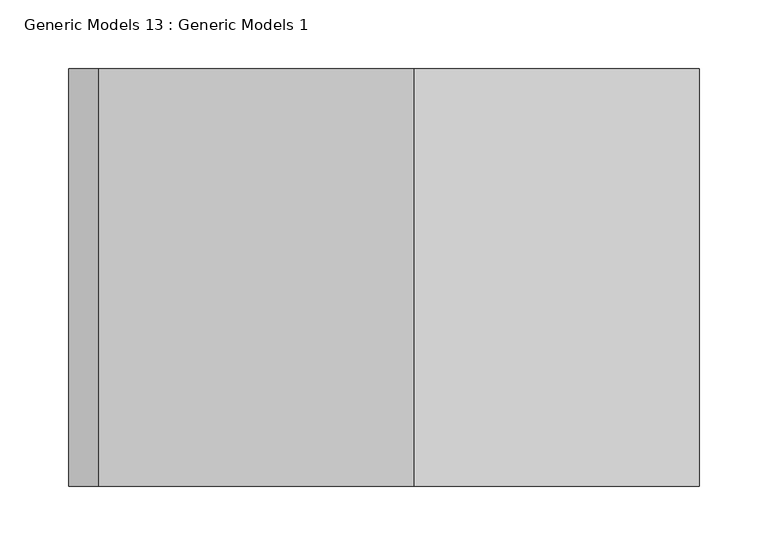
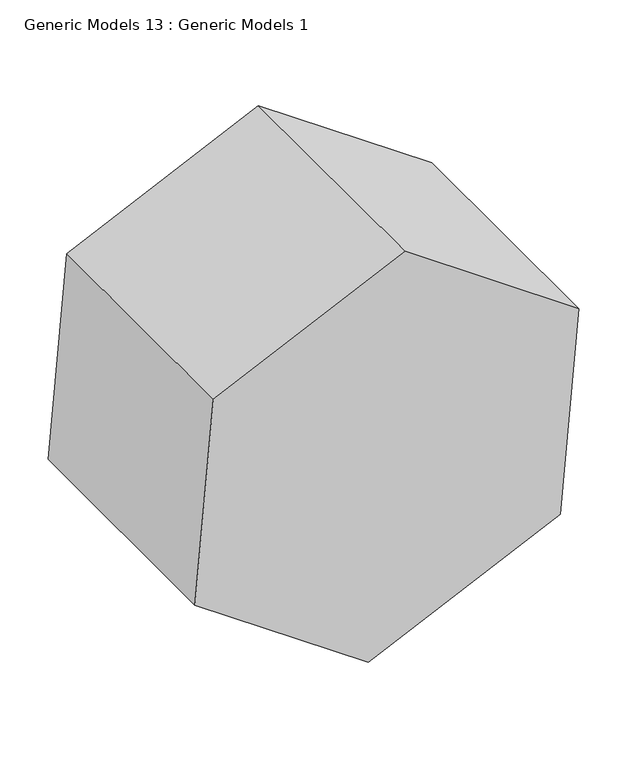
"""IFC4 building model written with IfcOpenShell, lengths in millimetres: proxy geometry, Generic Models 13 : Generic Models 1."""

from ifc_helpers import new_model, si_unit, frame, origin, place, context, project, spatial, polyline, outline, extrude, source, transform, mapped, element, save


def generic_models_13_generic_models_1_cefb3180(model_context):
    return source(origin(), model_context, "Body", "SweptSolid", [
        extrude(outline(polyline([(833.1013393, 3857.2920945), (978.7897542, 3649.2274753), (871.4447157, 3419.0252974), (618.4112624, 3396.8877387), (472.7228475, 3604.952358), (580.067886, 3835.1545359), (833.1013393, 3857.2920945)])), frame((0.0, -10720.3372434, 0.0), z_axis=(0.0, 1.0, 0.0), x_axis=(0.0, 0.0, 1.0)), (0.0, 0.0, 1.0), 304.8),
    ])


if __name__ == "__main__":
    model = new_model("IFC4")
    model_context = context("Model", 3, world=origin())
    ifc_project = project(units=[si_unit("LENGTHUNIT", "METRE", prefix="MILLI")], contexts=[model_context])
    site = spatial("IfcSite", under=ifc_project)
    building = spatial("IfcBuilding", under=site)
    placement = place(None, origin())
    generic_models_13_generic_models_1_shape = generic_models_13_generic_models_1_cefb3180(model_context)
    element("IfcBuildingElementProxy", 1, Name="Generic Models 13 : Generic Models 1", ObjectType="Generic Models 13 : Generic Models 1", at=placement, inside=building, context=model_context, shape_type="MappedRepresentation", body=[
        mapped(generic_models_13_generic_models_1_shape, transform((0.0, 0.0, 0.0), x_axis=(1.0, 0.0, 0.0), y_axis=(0.0, 1.0, 0.0), z_axis=(0.0, 0.0, 1.0))),
    ])
    save(model, "model.ifc")
